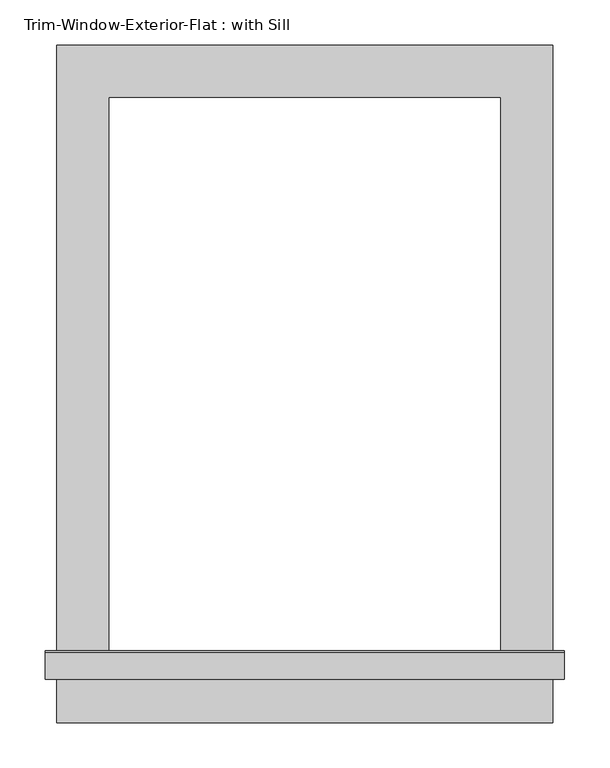
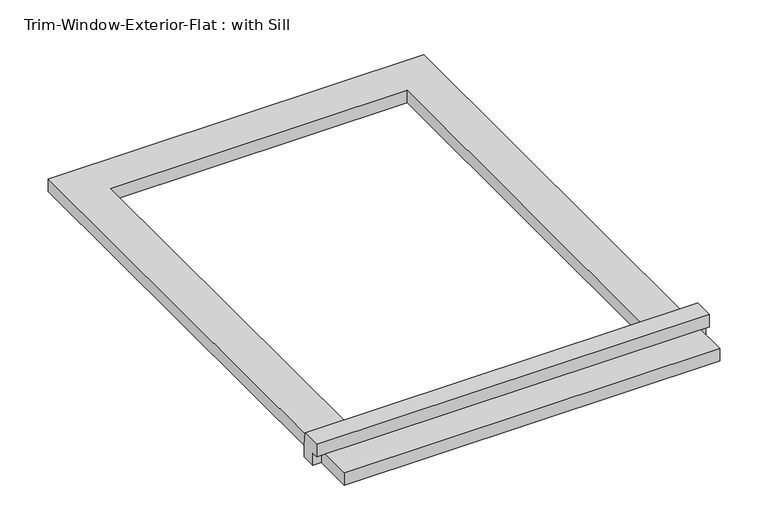
"""IFC4 building model written with IfcOpenShell, lengths in millimetres: proxy geometry, Trim-Window-Exterior-Flat : with Sill."""

from ifc_helpers import new_model, si_unit, frame, origin, origin_with_axes, place, context, project, spatial, polyline, outline, extrude, source, transform, mapped, element, save


def trim_window_exterior_flat_with_sill_e496db69(model_context):
    return source(origin(), model_context, "Body", "SweptSolid", [
        extrude(outline(polyline([(273.05, -631.7823709), (273.05, -688.9323709), (-273.05, -688.9323709), (-273.05, -631.7823709), (273.05, -631.7823709)])), origin_with_axes(), (0.0, 0.0, 1.0), 19.05),
        extrude(outline(polyline([(-641.35, 38.1), (-612.0580645, 38.1), (-609.6, 19.05), (-609.6, 0.0), (-631.7823709, 0.0), (-631.7823709, 19.05), (-641.35, 19.05), (-641.35, 38.1)])), frame((-285.75, 0.0, 0.0), z_axis=(1.0, 0.0, 0.0), x_axis=(0.0, 1.0, 0.0)), (0.0, 0.0, 1.0), 571.5),
        extrude(outline(polyline([(-273.05, 57.15), (273.05, 57.15), (273.05, -609.6), (215.9, -609.6), (215.9, 0.0), (-215.9, 0.0), (-215.9, -609.6), (-273.05, -609.6), (-273.05, 57.15)])), origin_with_axes(), (0.0, 0.0, 1.0), 19.05),
    ])


if __name__ == "__main__":
    model = new_model("IFC4")
    model_context = context("Model", 3, world=origin())
    ifc_project = project(units=[si_unit("LENGTHUNIT", "METRE", prefix="MILLI")], contexts=[model_context])
    site = spatial("IfcSite", under=ifc_project)
    building = spatial("IfcBuilding", under=site)
    placement = place(None, origin())
    trim_window_exterior_flat_with_sill_shape = trim_window_exterior_flat_with_sill_e496db69(model_context)
    element("IfcBuildingElementProxy", 1, Name="Trim-Window-Exterior-Flat : with Sill", ObjectType="Trim-Window-Exterior-Flat : with Sill", at=placement, inside=building, context=model_context, shape_type="MappedRepresentation", body=[
        mapped(trim_window_exterior_flat_with_sill_shape, transform((0.0, 0.0, 0.0), x_axis=(1.0, 0.0, 0.0), y_axis=(0.0, 1.0, 0.0), z_axis=(0.0, 0.0, 1.0))),
    ])
    save(model, "model.ifc")

# Revit data of these elements
# Type "Trim-Window-Exterior-Flat : with Sill"
#   Trim Width = 0' - 2 1/4"
#   Trim Thickness_Picture Frame = 0' - 1 1/4"
#   Trim Thickness_with Sill = 0' - 0 3/4"
#   Sill Thickness = 0' - 1 1/4"
#   Opening Width [instance default] = 2' - 0"
#   Opening Height [instance default] = 3' - 0"
#   Default Elevation = 4' - 0"
#   Sill = yes
#   Picture Frame = no
#   Trim Material [instance default] = none
# Element 1 (IfcBuildingElementProxy, "Trim-Window-Exterior-Flat : with Sill")
#   Opening Width = 1' - 5"
#   Opening Height = 2' - 0"
#   Trim Material = Clad - White
#   Materials on its faces: "Clad - White"
# Materials
#   "Clad - White": class "Wood", colour RGB 242 242 238, transparency 0, Cost = 0
